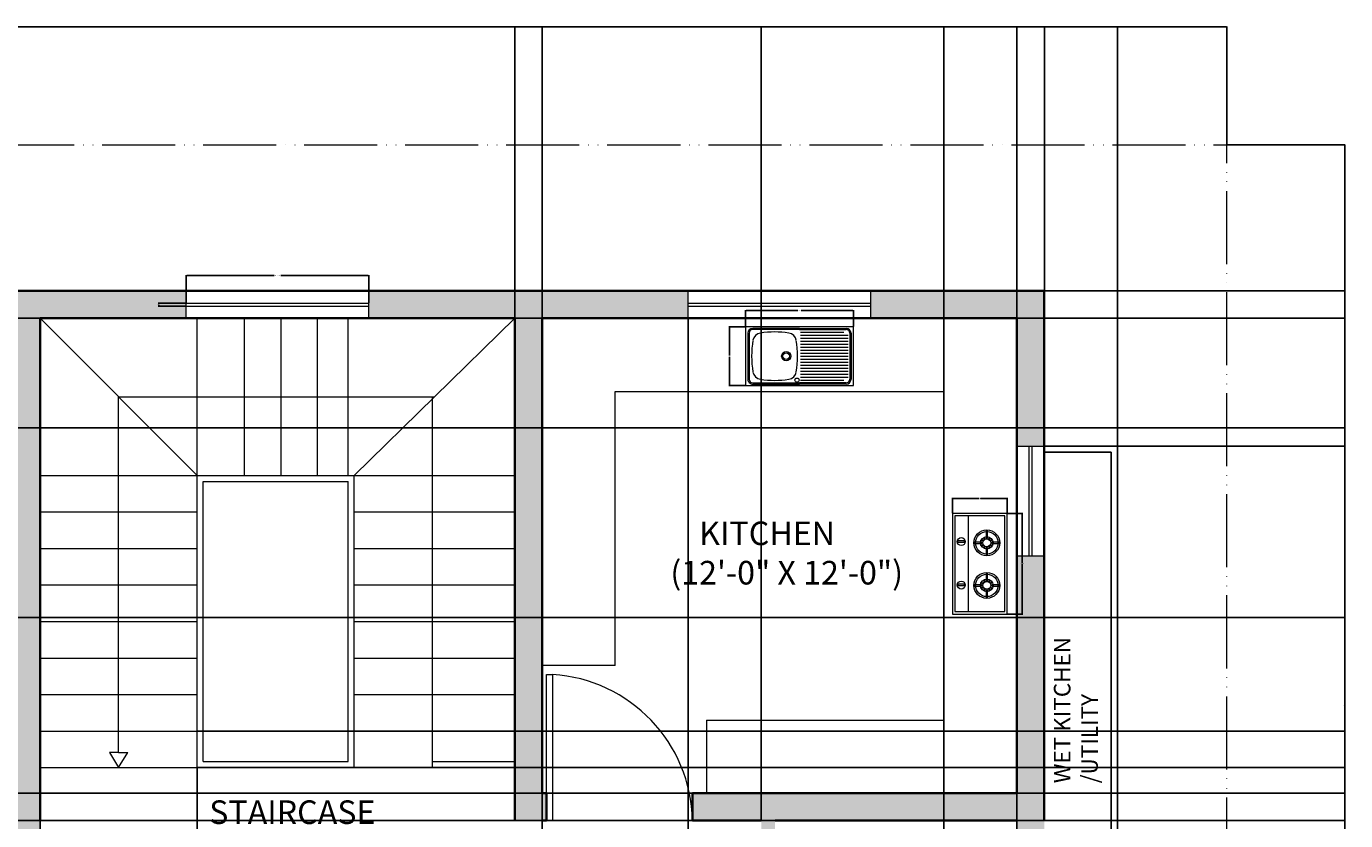
# Model space of a CAD drawing. Units: inches. Extents: x 2847 to 3693, y 1516 to 2098.
# Tile 6 of 6: x 3259 to 3693, y 1837 to 2098. Entities that reach past the tile are written whole.
import ezdxf

# ---------------------------------------------------------------- set-up
doc = ezdxf.new("R2010")
doc.units = ezdxf.units.IN
doc.linetypes.add('ACAD_ISO05W100', pattern=[33, 24, -3, 0, -3, 0, -3])
for name, color, linetype, lineweight in [('A-ANNO-DIMS', 2, 'Continuous', 18), ('A-AREA-IDEN', 7, 'Continuous', 18), ('A-DOOR', 3, 'Continuous', 18), ('A-EQPM', 9, 'Continuous', 18), ('A-FLOR', 7, 'Continuous', 25), ('A-FLOR-CASE', 8, 'Continuous', 18), ('A-FLOR-FIXT', 9, 'Continuous', 18), ('A-FLOR-STRS', 7, 'Continuous', 18), ('A-GLAZ', 4, 'Continuous', 18), ('A-WALL', 7, 'Continuous', 35), ('C-PROP', 7, 'ACAD_ISO05W100', 18)]:
    doc.layers.add(name, color=color, linetype=linetype, lineweight=lineweight)
doc.layers.add('A-WALL-PATT', color=251, linetype='Continuous', lineweight=13, true_color=0x636466)
doc.styles.get("Standard").update_dxf_attribs({"font": 'arial.ttf'})
doc.dimstyles.get("Standard").update_dxf_attribs({"dimtxt": 0.18, "dimasz": 0.18, "dimexe": 0.18, "dimexo": 0.0625, "dimgap": 0.09, "dimtad": 0, "dimtih": 1, "dimtoh": 1, "dimdec": 4, "dimzin": 0, "dimdsep": 46, "dimtxsty": 'Standard', "dimcen": 0.09, "dimadec": 0, "dimazin": 0, "dimtfac": 1, "dimtdec": 4, "dimtofl": 0, "dimtmove": 0, "dimatfit": 3, "dimfxl": 1, "dimtolj": 1, "dimtzin": 0, "dimarcsym": 0})

# ---------------------------------------------------------------- blocks, each defined once
blk = doc.blocks.new('A$C0C3933DC')
for p, q in [((0, 490), (0, 0)), ((900, 490), (0, 490)), ((60, 478), (450, 478)), ((60, 468), (450, 468)), ((441, 445), (81, 445)), ((841, 478), (450, 478)), ((841, 468), (450, 468)), ((900, 0), (900, 490)), ((20, 53), (20, 438)), ((30, 53), (30, 438)), ((441, 420), (45, 420)), ((441, 395), (45, 395)), ((441, 370), (45, 370)), ((441, 345), (45, 345)), ((871, 53), (871, 438)), ((881, 53), (881, 438)), ((441, 320), (45, 320)), ((441, 295), (45, 295)), ((441, 270), (45, 270)), ((441, 245), (45, 245)), ((441, 220), (45, 220)), ((441, 195), (45, 195)), ((441, 170), (45, 170)), ((441, 145), (45, 145)), ((441, 120), (45, 120)), ((0, 0), (900, 0)), ((441, 95), (45, 95)), ((441, 70), (45, 70)), ((450, 23), (60, 23)), ((450, 13), (60, 13)), ((441, 45), (81, 45)), ((450, 23), (841, 23)), ((450, 13), (841, 13))]:
    blk.add_line(p, q)
for centre, radius in [((471, 445), 17.5), ((561, 245), 38), ((561, 245), 27.5)]:
    blk.add_circle(centre, radius)
for centre, radius, start, end in [((60, 438), 40, 90, 180), ((60, 438), 30, 90, 180), ((658, -303), 750, 80.9213, 99.0787), ((841, 438), 40, 0, 90), ((841, 438), 30, 0, 90), ((1216, 245), 750, 169.8852, 190.1148), ((551, 364), 75, 99.0787, 169.8852), ((765, 364), 75, 10.1148, 80.9213), ((100, 245), 750, 349.8852, 10.1148), ((551, 126), 75, 190.1148, 260.9213), ((765, 126), 75, 279.0787, 349.8852), ((60, 53), 40, 180, 270), ((60, 53), 30, 180, 270), ((658, 793), 750, 260.9213, 279.0787), ((841, 53), 30, 270, 0), ((841, 53), 40, 270, 0)]:
    blk.add_arc(centre, radius, start, end)
blk = doc.blocks.new('A$C06E242FC')
for p, q in [((0, 456), (0, 456)), ((0, 456), (0, 0)), ((839, 456), (0, 456)), ((839, 456), (839, 456)), ((839, 0), (839, 456)), ((20, 436), (20, 436)), ((20, 436), (20, 20)), ((819, 436), (20, 436)), ((237, 411), (237, 356)), ((249, 411), (237, 411)), ((237, 356), (249, 356)), ((249, 356), (249, 411)), ((599, 411), (611, 411)), ((599, 411), (599, 356)), ((599, 356), (611, 356)), ((611, 356), (611, 411)), ((819, 436), (819, 436)), ((819, 20), (819, 436)), ((20, 324), (819, 324)), ((233, 273), (233, 214)), ((245, 273), (233, 273)), ((245, 214), (245, 273)), ((588, 273), (588, 214)), ((600, 273), (588, 273)), ((600, 214), (600, 273)), ((136, 176), (136, 164)), ((195, 176), (136, 176)), ((136, 164), (195, 164)), ((195, 164), (195, 176)), ((233, 214), (245, 214)), ((245, 126), (233, 126)), ((233, 126), (233, 67)), ((245, 67), (245, 126)), ((283, 176), (283, 164)), ((342, 176), (283, 176)), ((283, 164), (342, 164)), ((342, 164), (342, 176)), ((550, 176), (492, 176)), ((492, 176), (492, 164)), ((492, 164), (550, 164)), ((550, 164), (550, 176)), ((588, 214), (600, 214)), ((601, 126), (588, 126)), ((588, 126), (588, 67)), ((601, 67), (601, 126)), ((638, 176), (638, 164)), ((697, 176), (638, 176)), ((638, 164), (697, 164)), ((697, 164), (697, 176)), ((0, 0), (0, 0)), ((20, 20), (20, 20)), ((20, 20), (819, 20)), ((233, 67), (245, 67)), ((588, 67), (601, 67)), ((819, 20), (819, 20)), ((839, 0), (839, 0)), ((0, 0), (839, 0))]:
    blk.add_line(p, q)
for centre, radius in [((242, 383), 33.3), ((604, 383), 33.3), ((239, 170), 108), ((239, 170), 93.3), ((239, 170), 52.6), ((594, 170), 108), ((594, 170), 93.3), ((594, 170), 52.6), ((200, 170), 4.84), ((205, 189), 4.84), ((205, 151), 4.84), ((239, 170), 32.6), ((220, 204), 4.84), ((220, 136), 4.84), ((239, 209), 4.84), ((239, 131), 4.84), ((258, 204), 4.84), ((258, 136), 4.84), ((273, 189), 4.84), ((273, 151), 4.84), ((278, 170), 4.84), ((555, 170), 4.84), ((561, 189), 4.84), ((561, 151), 4.84), ((594, 170), 32.6), ((575, 204), 4.84), ((575, 136), 4.84), ((594, 209), 4.84), ((594, 131), 4.84), ((614, 204), 4.84), ((614, 136), 4.84), ((628, 189), 4.84), ((628, 151), 4.84), ((633, 170), 4.84)]:
    blk.add_circle(centre, radius)
blk = doc.blocks.new('WIN-GLAZ-60IN')
for p, q in [((0, 1), (60, 1)), ((0, 0), (60, 0))]:
    blk.add_line(p, q)
blk = doc.blocks.new('WIN-GLAZ-36IN')
for p, q in [((36, 1), (0, 1)), ((36, 0), (0, 0))]:
    blk.add_line(p, q)
blk = doc.blocks.new('*D15')
at = {"layer": 'A-ANNO-DIMS', "color": 0, "lineweight": -2, "transparency": 16777216}
for p, q in [((3311.85, 2007.18), (3311.85, 2016.3)), ((3312.03, 2016.12), (3340.73, 2016.12)), ((3371.67, 2016.12), (3342.96, 2016.12)), ((3371.85, 2007.18), (3371.85, 2016.3))]:
    blk.add_line(p, q, dxfattribs=at)
at = {"layer": 'A-ANNO-DIMS', "color": 0, "transparency": 16777216}
for points in [[(3312.03, 2016.15), (3312.03, 2016.09), (3311.85, 2016.12)], [(3371.67, 2016.15), (3371.67, 2016.09), (3371.85, 2016.12)]]:
    blk.add_solid(points, dxfattribs=at)
at = {"layer": 'Defpoints', "color": 0, "transparency": 16777216}
for p in [(3371.85, 2016.12), (3311.85, 2007.12), (3371.85, 2007.12)]:
    blk.add_point(p, dxfattribs=at)
at = {"layer": 'A-ANNO-DIMS', "color": 0, "transparency": 16777216, "insert": (3341.85, 2016.12), "char_height": 0.18, "attachment_point": 5}
blk.add_mtext('\\A1;WINDOW 60 TYP.', dxfattribs=at)
blk = doc.blocks.new('*D16')
at = {"layer": 'A-ANNO-DIMS', "color": 0, "lineweight": -2, "transparency": 16777216}
for p, q in [((3311.78, 2007.12), (3302.67, 2007.12)), ((3311.78, 2006.12), (3302.67, 2006.12)), ((3302.85, 2006.94), (3302.85, 2006.8)), ((3302.85, 2006.3), (3302.85, 2006.44))]:
    blk.add_line(p, q, dxfattribs=at)
at = {"layer": 'A-ANNO-DIMS', "color": 0, "transparency": 16777216}
for points in [[(3302.82, 2006.94), (3302.88, 2006.94), (3302.85, 2007.12)], [(3302.82, 2006.3), (3302.88, 2006.3), (3302.85, 2006.12)]]:
    blk.add_solid(points, dxfattribs=at)
at = {"layer": 'Defpoints', "color": 0, "transparency": 16777216}
for p in [(3302.85, 2007.12), (3311.85, 2007.12), (3311.85, 2006.12)]:
    blk.add_point(p, dxfattribs=at)
at = {"layer": 'A-ANNO-DIMS', "color": 0, "transparency": 16777216, "insert": (3302.85, 2006.62), "char_height": 0.18, "attachment_point": 5}
blk.add_mtext('\\A1;1 TYP.', dxfattribs=at)
blk = doc.blocks.new('*D31')
at = {"layer": 'A-ANNO-DIMS', "color": 0, "lineweight": -2, "transparency": 16777216}
for p, q in [((3495.68, 1999.38), (3495.68, 2004.81)), ((3495.86, 2004.63), (3512.85, 2004.63)), ((3530.94, 2004.63), (3513.95, 2004.63)), ((3531.12, 1999.38), (3531.12, 2004.81))]:
    blk.add_line(p, q, dxfattribs=at)
at = {"layer": 'A-ANNO-DIMS', "color": 0, "transparency": 16777216}
for points in [[(3495.86, 2004.66), (3495.86, 2004.6), (3495.68, 2004.63)], [(3530.94, 2004.66), (3530.94, 2004.6), (3531.12, 2004.63)]]:
    blk.add_solid(points, dxfattribs=at)
at = {"layer": 'Defpoints', "color": 0, "transparency": 16777216}
for p in [(3495.68, 2004.63), (3495.68, 1999.32), (3531.12, 1999.32)]:
    blk.add_point(p, dxfattribs=at)
at = {"layer": 'A-ANNO-DIMS', "color": 0, "transparency": 16777216, "insert": (3513.4, 2004.63), "char_height": 0.18, "attachment_point": 5}
blk.add_mtext('\\A1;SINK 35', dxfattribs=at)
blk = doc.blocks.new('*D32')
at = {"layer": 'A-ANNO-DIMS', "color": 0, "lineweight": -2, "transparency": 16777216}
for p, q in [((3495.62, 1999.32), (3490.19, 1999.32)), ((3490.37, 1999.14), (3490.37, 1989.85)), ((3490.37, 1980.21), (3490.37, 1989.49)), ((3495.62, 1980.03), (3490.19, 1980.03))]:
    blk.add_line(p, q, dxfattribs=at)
at = {"layer": 'A-ANNO-DIMS', "color": 0, "transparency": 16777216}
for points in [[(3490.34, 1999.14), (3490.4, 1999.14), (3490.37, 1999.32)], [(3490.34, 1980.21), (3490.4, 1980.21), (3490.37, 1980.03)]]:
    blk.add_solid(points, dxfattribs=at)
at = {"layer": 'Defpoints', "color": 0, "transparency": 16777216}
for p in [(3495.68, 1999.32), (3490.37, 1980.03), (3495.68, 1980.03)]:
    blk.add_point(p, dxfattribs=at)
at = {"layer": 'A-ANNO-DIMS', "color": 0, "transparency": 16777216, "insert": (3490.37, 1989.67), "char_height": 0.18, "attachment_point": 5}
blk.add_mtext('\\A1;19', dxfattribs=at)
blk = doc.blocks.new('*D33')
at = {"layer": 'A-ANNO-DIMS', "color": 0, "lineweight": -2, "transparency": 16777216}
for p, q in [((3581.7, 1938.02), (3586.78, 1938.02)), ((3586.6, 1937.84), (3586.6, 1921.68)), ((3586.6, 1905.15), (3586.6, 1921.31)), ((3581.7, 1904.97), (3586.78, 1904.97))]:
    blk.add_line(p, q, dxfattribs=at)
at = {"layer": 'A-ANNO-DIMS', "color": 0, "transparency": 16777216}
for points in [[(3586.57, 1937.84), (3586.63, 1937.84), (3586.6, 1938.02)], [(3586.57, 1905.15), (3586.63, 1905.15), (3586.6, 1904.97)]]:
    blk.add_solid(points, dxfattribs=at)
at = {"layer": 'Defpoints', "color": 0, "transparency": 16777216}
for p in [(3581.64, 1938.02), (3586.6, 1938.02), (3581.64, 1904.97)]:
    blk.add_point(p, dxfattribs=at)
at = {"layer": 'A-ANNO-DIMS', "color": 0, "transparency": 16777216, "insert": (3586.6, 1921.49), "char_height": 0.18, "attachment_point": 5}
blk.add_mtext('\\A1;COOKTOP 33', dxfattribs=at)
blk = doc.blocks.new('*D34')
at = {"layer": 'A-ANNO-DIMS', "color": 0, "lineweight": -2, "transparency": 16777216}
for p, q in [((3563.68, 1938.08), (3563.68, 1943.15)), ((3563.86, 1942.97), (3572.45, 1942.97)), ((3581.46, 1942.97), (3572.87, 1942.97)), ((3581.64, 1938.08), (3581.64, 1943.15))]:
    blk.add_line(p, q, dxfattribs=at)
at = {"layer": 'A-ANNO-DIMS', "color": 0, "transparency": 16777216}
for points in [[(3563.86, 1943), (3563.86, 1942.94), (3563.68, 1942.97)], [(3581.46, 1943), (3581.46, 1942.94), (3581.64, 1942.97)]]:
    blk.add_solid(points, dxfattribs=at)
at = {"layer": 'Defpoints', "color": 0, "transparency": 16777216}
for p in [(3563.68, 1942.97), (3563.68, 1938.02), (3581.64, 1938.02)]:
    blk.add_point(p, dxfattribs=at)
at = {"layer": 'A-ANNO-DIMS', "color": 0, "transparency": 16777216, "insert": (3572.66, 1942.97), "char_height": 0.18, "attachment_point": 5}
blk.add_mtext('\\A1;18', dxfattribs=at)
blk = doc.blocks.new('*D35')
at = {"layer": 'A-ANNO-DIMS', "color": 0, "lineweight": -2, "transparency": 16777216}
for p, q in [((2885.85, 2059.18), (2885.85, 2098)), ((2886.03, 2097.82), (3269.56, 2097.82)), ((3653.67, 2097.82), (3270.13, 2097.82)), ((3653.85, 2059.18), (3653.85, 2098))]:
    blk.add_line(p, q, dxfattribs=at)
at = {"layer": 'A-ANNO-DIMS', "color": 0, "transparency": 16777216}
for points in [[(2886.03, 2097.85), (2886.03, 2097.79), (2885.85, 2097.82)], [(3653.67, 2097.85), (3653.67, 2097.79), (3653.85, 2097.82)]]:
    blk.add_solid(points, dxfattribs=at)
at = {"layer": 'Defpoints', "color": 0, "transparency": 16777216}
for p in [(3653.85, 2097.82), (2885.85, 2059.12), (3653.85, 2059.12)]:
    blk.add_point(p, dxfattribs=at)
at = {"layer": 'A-ANNO-DIMS', "color": 0, "transparency": 16777216, "insert": (3269.85, 2097.82), "char_height": 0.18, "attachment_point": 5}
blk.add_mtext('\\A1;768', dxfattribs=at)
blk = doc.blocks.new('*D36')
at = {"layer": 'A-ANNO-DIMS', "color": 0, "lineweight": -2, "transparency": 16777216}
for p, q in [((3653.91, 2059.12), (3692.73, 2059.12)), ((3692.55, 2058.94), (3692.55, 1807.3)), ((3692.55, 1555.3), (3692.55, 1806.94)), ((3653.91, 1555.12), (3692.73, 1555.12))]:
    blk.add_line(p, q, dxfattribs=at)
at = {"layer": 'A-ANNO-DIMS', "color": 0, "transparency": 16777216}
for points in [[(3692.52, 2058.94), (3692.58, 2058.94), (3692.55, 2059.12)], [(3692.52, 1555.3), (3692.58, 1555.3), (3692.55, 1555.12)]]:
    blk.add_solid(points, dxfattribs=at)
at = {"layer": 'Defpoints', "color": 0, "transparency": 16777216}
for p in [(3653.85, 2059.12), (3692.55, 2059.12), (3653.85, 1555.12)]:
    blk.add_point(p, dxfattribs=at)
at = {"layer": 'A-ANNO-DIMS', "color": 0, "transparency": 16777216, "insert": (3692.55, 1807.12), "char_height": 0.18, "attachment_point": 5}
blk.add_mtext('\\A1;504', dxfattribs=at)
blk = doc.blocks.new('*D41')
at = {"layer": 'A-ANNO-DIMS', "color": 0, "lineweight": -2, "transparency": 16777216}
for p, q in [((3254.85, 2002.18), (3254.85, 2098)), ((3255.03, 2097.82), (3337.06, 2097.82)), ((3419.67, 2097.82), (3337.63, 2097.82)), ((3419.85, 2002.18), (3419.85, 2098))]:
    blk.add_line(p, q, dxfattribs=at)
at = {"layer": 'A-ANNO-DIMS', "color": 0, "transparency": 16777216}
for points in [[(3255.03, 2097.85), (3255.03, 2097.79), (3254.85, 2097.82)], [(3419.67, 2097.85), (3419.67, 2097.79), (3419.85, 2097.82)]]:
    blk.add_solid(points, dxfattribs=at)
at = {"layer": 'Defpoints', "color": 0, "transparency": 16777216}
for p in [(3419.85, 2097.82), (3254.85, 2002.12), (3419.85, 2002.12)]:
    blk.add_point(p, dxfattribs=at)
at = {"layer": 'A-ANNO-DIMS', "color": 0, "transparency": 16777216, "insert": (3337.35, 2097.82), "char_height": 0.18, "attachment_point": 5}
blk.add_mtext('\\A1;165', dxfattribs=at)
blk = doc.blocks.new('*D42')
at = {"layer": 'A-ANNO-DIMS', "color": 0, "lineweight": -2, "transparency": 16777216}
for p, q in [((3419.85, 2002.18), (3419.85, 2098)), ((3420.03, 2097.82), (3506.57, 2097.82)), ((3593.67, 2097.82), (3507.13, 2097.82)), ((3593.85, 2011.18), (3593.85, 2098))]:
    blk.add_line(p, q, dxfattribs=at)
at = {"layer": 'A-ANNO-DIMS', "color": 0, "transparency": 16777216}
for points in [[(3420.03, 2097.85), (3420.03, 2097.79), (3419.85, 2097.82)], [(3593.67, 2097.85), (3593.67, 2097.79), (3593.85, 2097.82)]]:
    blk.add_solid(points, dxfattribs=at)
at = {"layer": 'Defpoints', "color": 0, "transparency": 16777216}
for p in [(3593.85, 2097.82), (3593.85, 2011.12), (3419.85, 2002.12)]:
    blk.add_point(p, dxfattribs=at)
at = {"layer": 'A-ANNO-DIMS', "color": 0, "transparency": 16777216, "insert": (3506.85, 2097.82), "char_height": 0.18, "attachment_point": 5}
blk.add_mtext('\\A1;174', dxfattribs=at)
blk = doc.blocks.new('*D47')
at = {"layer": 'A-ANNO-DIMS', "color": 0, "lineweight": -2, "transparency": 16777216}
for p, q in [((3617.91, 1960.12), (3692.73, 1960.12)), ((3692.55, 1959.94), (3692.55, 1862.8)), ((3692.55, 1765.3), (3692.55, 1862.44)), ((3617.91, 1765.12), (3692.73, 1765.12))]:
    blk.add_line(p, q, dxfattribs=at)
at = {"layer": 'A-ANNO-DIMS', "color": 0, "transparency": 16777216}
for points in [[(3692.52, 1959.94), (3692.58, 1959.94), (3692.55, 1960.12)], [(3692.52, 1765.3), (3692.58, 1765.3), (3692.55, 1765.12)]]:
    blk.add_solid(points, dxfattribs=at)
at = {"layer": 'Defpoints', "color": 0, "transparency": 16777216}
for p in [(3617.85, 1960.12), (3692.55, 1960.12), (3617.85, 1765.12)]:
    blk.add_point(p, dxfattribs=at)
at = {"layer": 'A-ANNO-DIMS', "color": 0, "transparency": 16777216, "insert": (3692.55, 1862.62), "char_height": 0.18, "attachment_point": 5}
blk.add_mtext('\\A1;195', dxfattribs=at)
blk = doc.blocks.new('*D48')
at = {"layer": 'A-ANNO-DIMS', "color": 0, "lineweight": -2, "transparency": 16777216}
for p, q in [((3593.85, 1960.18), (3593.85, 2098)), ((3594.03, 2097.82), (3605.63, 2097.82)), ((3617.67, 2097.82), (3606.07, 2097.82)), ((3617.85, 1960.18), (3617.85, 2098))]:
    blk.add_line(p, q, dxfattribs=at)
at = {"layer": 'A-ANNO-DIMS', "color": 0, "transparency": 16777216}
for points in [[(3594.03, 2097.85), (3594.03, 2097.79), (3593.85, 2097.82)], [(3617.67, 2097.85), (3617.67, 2097.79), (3617.85, 2097.82)]]:
    blk.add_solid(points, dxfattribs=at)
at = {"layer": 'Defpoints', "color": 0, "transparency": 16777216}
for p in [(3617.85, 2097.82), (3593.85, 1960.12), (3617.85, 1960.12)]:
    blk.add_point(p, dxfattribs=at)
at = {"layer": 'A-ANNO-DIMS', "color": 0, "transparency": 16777216, "insert": (3605.85, 2097.82), "char_height": 0.18, "attachment_point": 5}
blk.add_mtext('\\A1;24', dxfattribs=at)
blk = doc.blocks.new('*D49')
at = {"layer": 'A-ANNO-DIMS', "color": 0, "lineweight": -2, "transparency": 16777216}
for p, q in [((3593.91, 2011.12), (3692.73, 2011.12)), ((3692.55, 2010.94), (3692.55, 1985.8)), ((3692.55, 1960.3), (3692.55, 1985.44)), ((3593.91, 1960.12), (3692.73, 1960.12))]:
    blk.add_line(p, q, dxfattribs=at)
at = {"layer": 'A-ANNO-DIMS', "color": 0, "transparency": 16777216}
for points in [[(3692.52, 2010.94), (3692.58, 2010.94), (3692.55, 2011.12)], [(3692.52, 1960.3), (3692.58, 1960.3), (3692.55, 1960.12)]]:
    blk.add_solid(points, dxfattribs=at)
at = {"layer": 'Defpoints', "color": 0, "transparency": 16777216}
for p in [(3593.85, 2011.12), (3692.55, 2011.12), (3593.85, 1960.12)]:
    blk.add_point(p, dxfattribs=at)
at = {"layer": 'A-ANNO-DIMS', "color": 0, "transparency": 16777216, "insert": (3692.55, 1985.62), "char_height": 0.18, "attachment_point": 5}
blk.add_mtext('\\A1;51', dxfattribs=at)
blk = doc.blocks.new('*D50')
at = {"layer": 'A-ANNO-DIMS', "color": 0, "lineweight": -2, "transparency": 16777216}
for p, q in [((2989.41, 2011.12), (3692.73, 2011.12)), ((3692.55, 2010.94), (3692.55, 1924.3)), ((3692.55, 1837.3), (3692.55, 1923.94)), ((2989.41, 1837.12), (3692.73, 1837.12))]:
    blk.add_line(p, q, dxfattribs=at)
at = {"layer": 'A-ANNO-DIMS', "color": 0, "transparency": 16777216}
for points in [[(3692.52, 2010.94), (3692.58, 2010.94), (3692.55, 2011.12)], [(3692.52, 1837.3), (3692.58, 1837.3), (3692.55, 1837.12)]]:
    blk.add_solid(points, dxfattribs=at)
at = {"layer": 'Defpoints', "color": 0, "transparency": 16777216}
for p in [(2989.35, 2011.12), (3692.55, 2011.12), (2989.35, 1837.12)]:
    blk.add_point(p, dxfattribs=at)
at = {"layer": 'A-ANNO-DIMS', "color": 0, "transparency": 16777216, "insert": (3692.55, 1924.12), "char_height": 0.18, "attachment_point": 5}
blk.add_mtext('\\A1;174', dxfattribs=at)
blk = doc.blocks.new('*D53')
at = {"layer": 'A-ANNO-DIMS', "color": 0, "lineweight": -2, "transparency": 16777216}
for p, q in [((3428.85, 1837.18), (3428.85, 2098)), ((3429.03, 2097.82), (3464.63, 2097.82)), ((3500.67, 2097.82), (3465.06, 2097.82)), ((3500.85, 1837.18), (3500.85, 2098))]:
    blk.add_line(p, q, dxfattribs=at)
at = {"layer": 'A-ANNO-DIMS', "color": 0, "transparency": 16777216}
for points in [[(3429.03, 2097.85), (3429.03, 2097.79), (3428.85, 2097.82)], [(3500.67, 2097.85), (3500.67, 2097.79), (3500.85, 2097.82)]]:
    blk.add_solid(points, dxfattribs=at)
at = {"layer": 'Defpoints', "color": 0, "transparency": 16777216}
for p in [(3500.85, 2097.82), (3428.85, 1837.12), (3500.85, 1837.12)]:
    blk.add_point(p, dxfattribs=at)
at = {"layer": 'A-ANNO-DIMS', "color": 0, "transparency": 16777216, "insert": (3464.85, 2097.82), "char_height": 0.18, "attachment_point": 5}
blk.add_mtext('\\A1;72', dxfattribs=at)
blk = doc.blocks.new('*D56')
at = {"layer": 'A-ANNO-DIMS', "color": 0, "lineweight": -2, "transparency": 16777216}
for p, q in [((3182.91, 1903.87), (3692.73, 1903.87)), ((3692.55, 1903.69), (3692.55, 1875.17)), ((3692.55, 1846.3), (3692.55, 1874.81)), ((3182.91, 1846.12), (3692.73, 1846.12))]:
    blk.add_line(p, q, dxfattribs=at)
at = {"layer": 'A-ANNO-DIMS', "color": 0, "transparency": 16777216}
for points in [[(3692.52, 1903.69), (3692.58, 1903.69), (3692.55, 1903.87)], [(3692.52, 1846.3), (3692.58, 1846.3), (3692.55, 1846.12)]]:
    blk.add_solid(points, dxfattribs=at)
at = {"layer": 'Defpoints', "color": 0, "transparency": 16777216}
for p in [(3182.85, 1903.87), (3692.55, 1903.87), (3182.85, 1846.12)]:
    blk.add_point(p, dxfattribs=at)
at = {"layer": 'A-ANNO-DIMS', "color": 0, "transparency": 16777216, "insert": (3692.55, 1874.99), "char_height": 0.18, "attachment_point": 5}
blk.add_mtext('\\A1;57.75', dxfattribs=at)
blk = doc.blocks.new('*D57')
at = {"layer": 'A-ANNO-DIMS', "color": 0, "lineweight": -2, "transparency": 16777216}
for p, q in [((3263.85, 1854.46), (3263.85, 1516.24)), ((3315.45, 1854.46), (3315.45, 1516.24)), ((3264.03, 1516.42), (3289.32, 1516.42)), ((3315.27, 1516.42), (3289.97, 1516.42))]:
    blk.add_line(p, q, dxfattribs=at)
at = {"layer": 'A-ANNO-DIMS', "color": 0, "transparency": 16777216}
for points in [[(3264.03, 1516.45), (3264.03, 1516.39), (3263.85, 1516.42)], [(3315.27, 1516.45), (3315.27, 1516.39), (3315.45, 1516.42)]]:
    blk.add_solid(points, dxfattribs=at)
at = {"layer": 'Defpoints', "color": 0, "transparency": 16777216}
for p in [(3263.85, 1854.52), (3315.45, 1854.52), (3315.45, 1516.42)]:
    blk.add_point(p, dxfattribs=at)
at = {"layer": 'A-ANNO-DIMS', "color": 0, "transparency": 16777216, "insert": (3289.65, 1516.42), "char_height": 0.18, "attachment_point": 5}
blk.add_mtext('\\A1;51.6', dxfattribs=at)
blk = doc.blocks.new('*D66')
at = {"layer": 'A-ANNO-DIMS', "color": 0, "lineweight": -2, "transparency": 16777216}
for p, q in [((3419.91, 2002.12), (3692.73, 2002.12)), ((3692.55, 2001.94), (3692.55, 1928.5)), ((3692.55, 1854.7), (3692.55, 1928.14)), ((3419.91, 1854.52), (3692.73, 1854.52))]:
    blk.add_line(p, q, dxfattribs=at)
at = {"layer": 'A-ANNO-DIMS', "color": 0, "transparency": 16777216}
for points in [[(3692.52, 2001.94), (3692.58, 2001.94), (3692.55, 2002.12)], [(3692.52, 1854.7), (3692.58, 1854.7), (3692.55, 1854.52)]]:
    blk.add_solid(points, dxfattribs=at)
at = {"layer": 'Defpoints', "color": 0, "transparency": 16777216}
for p in [(3419.85, 2002.12), (3419.85, 1854.52), (3692.55, 1854.52)]:
    blk.add_point(p, dxfattribs=at)
at = {"layer": 'A-ANNO-DIMS', "color": 0, "transparency": 16777216, "insert": (3692.55, 1928.32), "char_height": 0.18, "attachment_point": 5}
blk.add_mtext('\\A1;147.6', dxfattribs=at)
blk = doc.blocks.new('*D67')
at = {"layer": 'A-ANNO-DIMS', "color": 0, "lineweight": -2, "transparency": 16777216}
for p, q in [((3428.85, 2002.06), (3428.85, 1516.24)), ((3476.85, 2002.06), (3476.85, 1516.24)), ((3429.03, 1516.42), (3452.62, 1516.42)), ((3476.67, 1516.42), (3453.07, 1516.42))]:
    blk.add_line(p, q, dxfattribs=at)
at = {"layer": 'A-ANNO-DIMS', "color": 0, "transparency": 16777216}
for points in [[(3429.03, 1516.45), (3429.03, 1516.39), (3428.85, 1516.42)], [(3476.67, 1516.45), (3476.67, 1516.39), (3476.85, 1516.42)]]:
    blk.add_solid(points, dxfattribs=at)
at = {"layer": 'Defpoints', "color": 0, "transparency": 16777216}
for p in [(3428.85, 2002.12), (3476.85, 2002.12), (3476.85, 1516.42)]:
    blk.add_point(p, dxfattribs=at)
at = {"layer": 'A-ANNO-DIMS', "color": 0, "transparency": 16777216, "insert": (3452.85, 1516.42), "char_height": 0.18, "attachment_point": 5}
blk.add_mtext('\\A1;48', dxfattribs=at)
blk = doc.blocks.new('*D68')
at = {"layer": 'A-ANNO-DIMS', "color": 0, "lineweight": -2, "transparency": 16777216}
for p, q in [((3560.85, 1624.18), (3560.85, 2098)), ((3561.03, 2097.82), (3572.63, 2097.82)), ((3584.67, 2097.82), (3573.07, 2097.82)), ((3584.85, 1600.18), (3584.85, 2098))]:
    blk.add_line(p, q, dxfattribs=at)
at = {"layer": 'A-ANNO-DIMS', "color": 0, "transparency": 16777216}
for points in [[(3561.03, 2097.85), (3561.03, 2097.79), (3560.85, 2097.82)], [(3584.67, 2097.85), (3584.67, 2097.79), (3584.85, 2097.82)]]:
    blk.add_solid(points, dxfattribs=at)
at = {"layer": 'Defpoints', "color": 0, "transparency": 16777216}
for p in [(3560.85, 2097.82), (3560.85, 1624.12), (3584.85, 1600.12)]:
    blk.add_point(p, dxfattribs=at)
at = {"layer": 'A-ANNO-DIMS', "color": 0, "transparency": 16777216, "insert": (3572.85, 2097.82), "char_height": 0.18, "attachment_point": 5}
blk.add_mtext('\\A1;24', dxfattribs=at)
blk = doc.blocks.new('*D73')
at = {"layer": 'A-ANNO-DIMS', "color": 0, "lineweight": -2, "transparency": 16777216}
for p, q in [((3315.51, 1866.52), (3692.73, 1866.52)), ((3692.55, 1866.34), (3692.55, 1860.7)), ((3692.55, 1854.7), (3692.55, 1860.34)), ((3315.51, 1854.52), (3692.73, 1854.52))]:
    blk.add_line(p, q, dxfattribs=at)
at = {"layer": 'A-ANNO-DIMS', "color": 0, "transparency": 16777216}
for points in [[(3692.52, 1866.34), (3692.58, 1866.34), (3692.55, 1866.52)], [(3692.52, 1854.7), (3692.58, 1854.7), (3692.55, 1854.52)]]:
    blk.add_solid(points, dxfattribs=at)
at = {"layer": 'Defpoints', "color": 0, "transparency": 16777216}
for p in [(3315.45, 1866.52), (3692.55, 1866.52), (3315.45, 1854.52)]:
    blk.add_point(p, dxfattribs=at)
at = {"layer": 'A-ANNO-DIMS', "color": 0, "transparency": 16777216, "insert": (3692.55, 1860.52), "char_height": 0.18, "attachment_point": 5}
blk.add_mtext('\\A1;12', dxfattribs=at)
blk = doc.blocks.new('*D79')
at = {"layer": 'A-ANNO-DIMS', "color": 0, "lineweight": -2, "transparency": 16777216}
for p, q in [((3182.91, 2002.12), (3692.73, 2002.12)), ((3692.55, 2001.94), (3692.55, 1984.3)), ((3692.55, 1966.3), (3692.55, 1983.94)), ((3182.91, 1966.12), (3692.73, 1966.12))]:
    blk.add_line(p, q, dxfattribs=at)
at = {"layer": 'A-ANNO-DIMS', "color": 0, "transparency": 16777216}
for points in [[(3692.52, 2001.94), (3692.58, 2001.94), (3692.55, 2002.12)], [(3692.52, 1966.3), (3692.58, 1966.3), (3692.55, 1966.12)]]:
    blk.add_solid(points, dxfattribs=at)
at = {"layer": 'Defpoints', "color": 0, "transparency": 16777216}
for p in [(3182.85, 2002.12), (3692.55, 2002.12), (3182.85, 1966.12)]:
    blk.add_point(p, dxfattribs=at)
at = {"layer": 'A-ANNO-DIMS', "color": 0, "transparency": 16777216, "insert": (3692.55, 1984.12), "char_height": 0.18, "attachment_point": 5}
blk.add_mtext('\\A1;36', dxfattribs=at)

msp = doc.modelspace()

# ---------------------------------------------------------------- hatches: boundary and pattern name
at = {"layer": 'A-WALL-PATT'}
h = msp.add_hatch(color=256, dxfattribs=at)
h.dxf.hatch_style = 1
h.paths.add_polyline_path([(2998.3457, 2002.118), (3178.3457, 2002.118), (3178.3457, 1944.368, -0.0341147), (3182.8457, 1944.4698), (3182.8457, 2002.118), (3200.8457, 2002.118), (3200.8457, 2011.118), (2989.3457, 2011.118), (2989.3457, 1960.118), (2998.3457, 1960.118)])
h.paths.add_polyline_path([(2998.3457, 1888.118), (2989.3457, 1888.118), (2989.3457, 1837.118), (3089.8457, 1837.118), (3089.8457, 1778.618), (3098.8457, 1778.618), (3098.8457, 1837.118), (3130.3457, 1837.118, -0.05293254), (3130.1282, 1846.118), (2998.3457, 1846.118)])
h.paths.add_polyline_path([(3263.8457, 2002.118), (3311.8457, 2002.118), (3311.8457, 2011.118), (3263.8457, 2011.118), (3236.8457, 2011.118), (3236.8457, 2002.118), (3254.8457, 2002.118), (3254.8457, 1908.368), (3182.8457, 1908.368), (3178.3457, 1908.368), (3178.3457, 1886.993), (3182.8457, 1886.993), (3182.8457, 1903.868), (3254.8457, 1903.868), (3254.8457, 1846.118), (3182.8457, 1846.118), (3182.8457, 1850.993), (3178.3457, 1850.993), (3178.3457, 1837.118), (3254.8457, 1837.118), (3254.8457, 1790.618), (3263.8457, 1790.618), (3263.8457, 1837.118)])
h.paths.add_polyline_path([(2930.8457, 1837.118), (2921.8457, 1837.118), (2921.8457, 1828.118), (2930.8457, 1828.118)])
h.paths.add_polyline_path([(2930.8457, 1600.118), (2921.8457, 1600.118), (2921.8457, 1591.118), (2930.8457, 1591.118)])
h.paths.add_polyline_path([(3098.8457, 1658.618), (3089.8457, 1658.618), (3089.8457, 1591.118), (3140.8457, 1591.118), (3140.8457, 1600.118), (3098.8457, 1600.118)])
h.paths.add_polyline_path([(3305.8457, 1600.118), (3263.8457, 1600.118), (3263.8457, 1646.618), (3254.8457, 1646.618), (3254.8457, 1600.118), (3212.8457, 1600.118), (3212.8457, 1591.118), (3254.8457, 1591.118), (3305.8457, 1591.118)])
h.paths.add_polyline_path([(3470.8457, 1600.118), (3428.8457, 1600.118), (3428.8457, 1756.118), (3430.26, 1756.118), (3430.26, 1765.118), (3428.8457, 1765.118), (3419.8457, 1765.118), (3419.8457, 1600.118), (3377.8457, 1600.118), (3377.8457, 1591.118), (3470.8457, 1591.118)])
h.paths.add_polyline_path([(3593.8457, 1642.118), (3584.8457, 1642.118), (3584.8457, 1600.118), (3542.8457, 1600.118), (3542.8457, 1591.118), (3593.8457, 1591.118)])
h.paths.add_polyline_path([(3593.8457, 1796.083), (3584.8457, 1796.083), (3584.8457, 1765.118), (3505.3457, 1765.118), (3505.3457, 1837.118), (3584.8457, 1837.118), (3584.8457, 1832.083), (3593.8457, 1832.083), (3593.8457, 1837.118), (3593.8457, 1924.118), (3584.8457, 1924.118), (3584.8457, 1846.118), (3478.26, 1846.118), (3478.26, 1837.118), (3500.8457, 1837.118), (3500.8457, 1765.118), (3478.26, 1765.118, -0.03536449), (3478.26, 1758.7816), (3478.26, 1756.118), (3584.8457, 1756.118), (3584.8457, 1714.118), (3593.8457, 1714.118)])
h.paths.add_polyline_path([(3593.8457, 2011.118), (3536.8457, 2011.118), (3536.8457, 2002.118), (3584.8457, 2002.118), (3584.8457, 1960.118), (3593.8457, 1960.118)])
h.paths.add_polyline_path([(3476.8457, 2011.118), (3371.8457, 2011.118), (3371.8457, 2002.118), (3419.8457, 2002.118), (3419.8457, 1837.118), (3428.8457, 1837.118), (3430.26, 1837.118), (3430.26, 1846.118), (3428.8457, 1846.118), (3428.8457, 2002.118), (3476.8457, 2002.118)])

# ---------------------------------------------------------------- linework, layer by layer
at = {"layer": 'A-DOOR'}
for p, q in [((3430.26, 1837.118), (3430.26, 1885.118)), ((3430.26, 1885.118), (3432.26, 1885.118)), ((3432.26, 1885.118), (3432.26, 1837.118)), ((3432.26, 1837.118), (3430.26, 1837.118))]:
    msp.add_line(p, q, dxfattribs=at)
msp.add_arc((3429.1627, 1836.1081), 49.1076, 1.178343, 86.383906, dxfattribs=at)
at = {"layer": 'A-FLOR'}
for p, q in [((3617.8457, 1960.118), (3593.8457, 1960.118)), ((3617.8457, 1765.118), (3617.8457, 1960.118)), ((3615.8457, 1958.118), (3593.8457, 1958.118)), ((3615.8457, 1767.118), (3615.8457, 1958.118))]:
    msp.add_line(p, q, dxfattribs=at)
at = {"layer": 'A-FLOR-CASE'}
for p, q in [((3452.8457, 1978.118), (3560.8457, 1978.118)), ((3452.8457, 1888.118), (3452.8457, 1978.118)), ((3560.8457, 1870.118), (3560.8457, 1978.118)), ((3452.8457, 1888.118), (3428.8457, 1888.118)), ((3482.8457, 1870.118), (3560.8457, 1870.118)), ((3482.8457, 1870.118), (3482.8457, 1846.118))]:
    msp.add_line(p, q, dxfattribs=at)
at = {"layer": 'A-FLOR-STRS'}
for p, q in [((3315.4457, 1950.518), (3263.8457, 2002.118)), ((3315.4457, 1854.518), (3315.4457, 2002.118)), ((3331.0457, 1950.518), (3331.0457, 2002.118)), ((3343.0457, 1950.518), (3343.0457, 2002.118)), ((3355.0457, 1950.518), (3355.0457, 2002.118)), ((3365.0457, 1950.518), (3365.0457, 2002.118)), ((3367.0457, 1950.518), (3419.8457, 2002.118)), ((3289.6457, 1976.318), (3393.4457, 1976.318)), ((3289.6457, 1859.518), (3289.6457, 1976.318)), ((3392.8457, 1854.518), (3392.8457, 1976.318)), ((3263.8457, 1950.518), (3419.8457, 1950.518)), ((3317.4457, 1856.518), (3317.4457, 1948.518)), ((3317.4457, 1948.518), (3365.0457, 1948.518)), ((3365.0457, 1856.518), (3365.0457, 1948.518)), ((3367.0457, 1854.518), (3367.0457, 1950.518)), ((3263.8457, 1938.518), (3315.4457, 1938.518)), ((3367.0457, 1938.518), (3419.8457, 1938.518)), ((3263.8457, 1926.518), (3315.4457, 1926.518)), ((3367.0457, 1926.518), (3419.8457, 1926.518)), ((3263.8457, 1914.518), (3315.4457, 1914.518)), ((3367.0457, 1914.518), (3419.8457, 1914.518)), ((3263.8457, 1902.518), (3315.4457, 1902.518)), ((3367.0457, 1902.518), (3419.8457, 1902.518)), ((3263.8457, 1890.518), (3315.4457, 1890.518)), ((3367.0457, 1890.518), (3419.8457, 1890.518)), ((3263.8457, 1878.518), (3315.4457, 1878.518)), ((3367.0457, 1878.518), (3419.8457, 1878.518)), ((3263.8457, 1866.518), (3315.4457, 1866.518)), ((3367.0457, 1866.518), (3419.8457, 1866.518)), ((3289.6457, 1859.518), (3286.6457, 1859.518)), ((3286.6457, 1859.518), (3289.6457, 1854.518)), ((3289.6457, 1859.518), (3292.6457, 1859.518)), ((3289.6457, 1854.518), (3292.6457, 1859.518)), ((3317.4457, 1856.518), (3365.0457, 1856.518)), ((3392.8457, 1856.518), (3419.8457, 1856.518)), ((3263.8457, 1854.518), (3419.8457, 1854.518))]:
    msp.add_line(p, q, dxfattribs=at)
at = {"layer": 'A-GLAZ'}
for p, q in [((3311.8457, 2002.118), (3311.8457, 2011.118)), ((3371.8457, 2002.118), (3371.8457, 2011.118)), ((3476.8457, 2002.118), (3476.8457, 2011.118)), ((3536.8457, 2002.118), (3536.8457, 2011.118)), ((3341.8457, 2002.118), (3341.8457, 2002.118)), ((3584.8457, 1960.118), (3593.8457, 1960.118)), ((3584.8457, 1924.118), (3593.8457, 1924.118))]:
    msp.add_line(p, q, dxfattribs=at)
at = {"layer": 'A-WALL'}
for p, q in [((2989.3457, 2011.118), (3263.8457, 2011.118)), ((3263.8457, 2011.118), (3593.8457, 2011.118)), ((3593.8457, 1837.118), (3593.8457, 2011.118)), ((3263.8457, 1837.118), (3263.8457, 2002.118)), ((3263.8457, 2002.118), (3419.8457, 2002.118)), ((3419.8457, 1837.118), (3419.8457, 2002.118)), ((3428.8457, 1846.118), (3428.8457, 2002.118)), ((3428.8457, 2002.118), (3584.8457, 2002.118)), ((3584.8457, 1846.118), (3584.8457, 2002.118)), ((3428.8457, 1846.118), (3430.26, 1846.118)), ((3430.26, 1846.118), (3430.26, 1837.118)), ((3478.26, 1846.118), (3478.26, 1837.118)), ((3478.26, 1846.118), (3584.8457, 1846.118)), ((3428.8457, 1837.118), (3430.26, 1837.118)), ((3478.26, 1837.118), (3500.8457, 1837.118)), ((3505.3457, 1837.118), (3584.8457, 1837.118))]:
    msp.add_line(p, q, dxfattribs=at)
at = {"layer": 'C-PROP'}
for p in [(2885.8457, 2059.118), (3653.8457, 1555.118)]:
    msp.add_line(p, (3653.8457, 2059.118), dxfattribs=at)

# ---------------------------------------------------------------- block references
at = {"layer": 'A-EQPM', "xscale": 0.0393700787401575, "yscale": 0.0393700787401575, "zscale": 0.0393700787401575, "rotation": 90}
msp.add_blockref('A$C06E242FC', (3581.6387, 1904.9705), dxfattribs=at)
at = {"layer": 'A-FLOR-FIXT', "xscale": 0.0393700787401575, "yscale": 0.0393700787401575, "zscale": 0.0393700787401575, "rotation": 180.0000000000002}
msp.add_blockref('A$C0C3933DC', (3531.1169, 1999.3187), dxfattribs=at)
at = {"layer": 'A-GLAZ'}
for p in [(3311.846, 2006.118), (3476.846, 2006.118)]:
    msp.add_blockref('WIN-GLAZ-60IN', p, dxfattribs=at)
at = {"layer": 'A-GLAZ', "rotation": 270}
msp.add_blockref('WIN-GLAZ-36IN', (3588.8457, 1960.1177), dxfattribs=at)

# ---------------------------------------------------------------- texts
at = {"layer": 'A-AREA-IDEN', "char_height": 7.756994, "attachment_point": 1}
for s, insert in [('    KITCHEN\\P(12\'-0" X 12\'-0")', (3470.958, 1935.3608)), ('STAIRCASE\\P(8\'-0" WIDE)', (3319.4178, 1843.7621))]:
    msp.add_mtext_dynamic_manual_height_columns(s, width=207.07675, gutter_width=38.785, heights=[0], dxfattribs=dict(at, insert=insert))
at = {"layer": 'A-AREA-IDEN', "insert": (3597.0024, 1849.3848), "char_height": 5.413701, "attachment_point": 1, "rotation": 90}
msp.add_mtext_dynamic_manual_height_columns('WET KITCHEN\\P/UTILITY', width=144.521402, gutter_width=27.0685, heights=[0], dxfattribs=at)

# ---------------------------------------------------------------- dimensions: what is measured, and where the dimension line sits
at = {"layer": 'A-ANNO-DIMS'}
for base, p1, p2, override, picture, middle in [((3653.8457, 2097.818), (2885.8457, 2059.118), (3653.8457, 2059.118), {"dimdec": 0, "dimlfac": 1, "dimrnd": 0, "dimzin": 0, "dimdsep": 46, "dimlunit": 2}, '*D35', (3269.8457, 2097.818)), ((3419.8457, 2097.818), (3254.8457, 2002.118), (3419.8457, 2002.118), {"dimdec": 0, "dimlfac": 1, "dimrnd": 0, "dimzin": 0, "dimdsep": 46, "dimlunit": 2}, '*D41', (3337.3457, 2097.818)), ((3593.8457, 2097.818), (3419.8457, 2002.118), (3593.8457, 2011.118), {"dimdec": 0, "dimlfac": 1, "dimrnd": 0, "dimzin": 0, "dimdsep": 46, "dimlunit": 2}, '*D42', (3506.8457, 2097.818)), ((3500.8457, 2097.818), (3428.8457, 1837.118), (3500.8457, 1837.118), {"dimdec": 0, "dimlfac": 1, "dimrnd": 0, "dimzin": 0, "dimdsep": 46, "dimlunit": 2}, '*D53', (3464.8457, 2097.818)), ((3560.8457, 2097.818), (3584.8457, 1600.118), (3560.8457, 1624.118), {"dimdec": 0, "dimlfac": 1, "dimrnd": 0, "dimzin": 0, "dimdsep": 46, "dimlunit": 2}, '*D68', (3572.8457, 2097.818)), ((3617.8457, 2097.818), (3593.8457, 1960.118), (3617.8457, 1960.118), {"dimdec": 0, "dimlfac": 1, "dimrnd": 0, "dimzin": 0, "dimdsep": 46, "dimlunit": 2}, '*D48', (3605.8457, 2097.818)), ((3476.8457, 1516.418), (3428.8457, 2002.118), (3476.8457, 2002.118), {"dimdec": 0, "dimlfac": 1, "dimrnd": 0, "dimzin": 0, "dimdsep": 46, "dimlunit": 2}, '*D67', (3452.8457, 1516.418)), ((3315.4457, 1516.418), (3263.8457, 1854.518), (3315.4457, 1854.518), {"dimdec": 1, "dimlfac": 1, "dimrnd": 0, "dimzin": 0, "dimdsep": 46, "dimlunit": 2}, '*D57', (3289.6457, 1516.418))]:
    dim = msp.add_linear_dim(base=base, p1=p1, p2=p2, dimstyle='Standard', override=override, dxfattribs=at)
    dim.commit()
    dim.dimension.update_dxf_attribs({"geometry": picture, "text_midpoint": middle})
for base, p1, p2, angle, override, picture, middle in [((3692.5457, 2059.118), (3653.8457, 1555.118), (3653.8457, 2059.118), 90, {"dimdec": 0, "dimlfac": 1, "dimrnd": 0, "dimzin": 0, "dimdsep": 46, "dimlunit": 2}, '*D36', (3692.5457, 1807.118)), ((3692.5457, 2011.118), (2989.3457, 1837.118), (2989.3457, 2011.118), 90, {"dimdec": 0, "dimlfac": 1, "dimrnd": 0, "dimzin": 0, "dimdsep": 46, "dimlunit": 2}, '*D50', (3692.5457, 1924.118)), ((3692.5457, 2011.118), (3593.8457, 1960.118), (3593.8457, 2011.118), 90, {"dimdec": 0, "dimlfac": 1, "dimrnd": 0, "dimzin": 0, "dimdsep": 46, "dimlunit": 2}, '*D49', (3692.5457, 1985.618)), ((3692.5457, 2002.118), (3182.8457, 1966.118), (3182.8457, 2002.118), 90, {"dimdec": 0, "dimlfac": 1, "dimrnd": 0, "dimzin": 0, "dimdsep": 46, "dimlunit": 2}, '*D79', (3692.5457, 1984.118)), ((3692.5457, 1854.518), (3419.8457, 2002.118), (3419.8457, 1854.518), 90, {"dimdec": 1, "dimlfac": 1, "dimrnd": 0, "dimzin": 0, "dimdsep": 46, "dimlunit": 2}, '*D66', (3692.5457, 1928.318)), ((3490.3689, 1980.0273), (3495.6838, 1999.3187), (3495.6838, 1980.0273), 270, {"dimdec": 0, "dimlfac": 1, "dimrnd": 0, "dimzin": 0, "dimdsep": 46, "dimlunit": 2}, '*D32', (3490.3689, 1989.673)), ((3692.5457, 1960.118), (3617.8457, 1765.118), (3617.8457, 1960.118), 90, {"dimdec": 0, "dimlfac": 1, "dimrnd": 0, "dimzin": 0, "dimdsep": 46, "dimlunit": 2}, '*D47', (3692.5457, 1862.618)), ((3563.6815, 1942.9747), (3581.6387, 1938.0176), (3563.6815, 1938.0176), 180, {"dimdec": 0, "dimlfac": 1, "dimrnd": 0, "dimzin": 0, "dimdsep": 46, "dimlunit": 2}, '*D34', (3572.6601, 1942.9747)), ((3692.5457, 1903.868), (3182.8457, 1846.118), (3182.8457, 1903.868), 90, {"dimdec": 2, "dimlfac": 1, "dimrnd": 0, "dimzin": 0, "dimdsep": 46, "dimlunit": 2}, '*D56', (3692.5457, 1874.993)), ((3692.5457, 1866.518), (3315.4457, 1854.518), (3315.4457, 1866.518), 90, {"dimdec": 0, "dimlfac": 1, "dimrnd": 0, "dimzin": 0, "dimdsep": 46, "dimlunit": 2}, '*D73', (3692.5457, 1860.518))]:
    dim = msp.add_linear_dim(base=base, p1=p1, p2=p2, angle=angle, dimstyle='Standard', override=override, dxfattribs=at)
    dim.commit()
    dim.dimension.update_dxf_attribs({"geometry": picture, "text_midpoint": middle})
dim = msp.add_linear_dim(base=(3371.8457, 2016.118), p1=(3311.8457, 2007.118), p2=(3371.8457, 2007.118), text='WINDOW <> TYP.', dimstyle='Standard', override={"dimdec": 0, "dimlfac": 1, "dimrnd": 0, "dimzin": 0, "dimdsep": 46, "dimlunit": 2}, dxfattribs=at)
dim.commit()
dim.dimension.update_dxf_attribs({"geometry": '*D15', "text_midpoint": (3341.8457, 2016.118)})
for base, p1, p2, angle, text, picture, middle in [((3302.8457, 2007.118), (3311.8457, 2006.118), (3311.8457, 2007.118), 90, '<> TYP.', '*D16', (3302.8457, 2006.618)), ((3495.6838, 2004.6336), (3531.1169, 1999.3187), (3495.6838, 1999.3187), 180, 'SINK <>', '*D31', (3513.4004, 2004.6336)), ((3586.5958, 1938.0176), (3581.6387, 1904.9705), (3581.6387, 1938.0176), 90, 'COOKTOP <>', '*D33', (3586.5958, 1921.4941))]:
    dim = msp.add_linear_dim(base=base, p1=p1, p2=p2, angle=angle, text=text, dimstyle='Standard', override={"dimdec": 0, "dimlfac": 1, "dimrnd": 0, "dimzin": 0, "dimdsep": 46, "dimlunit": 2}, dxfattribs=at)
    dim.commit()
    dim.dimension.update_dxf_attribs({"geometry": picture, "text_midpoint": middle})

doc.saveas('drawing.dxf')
